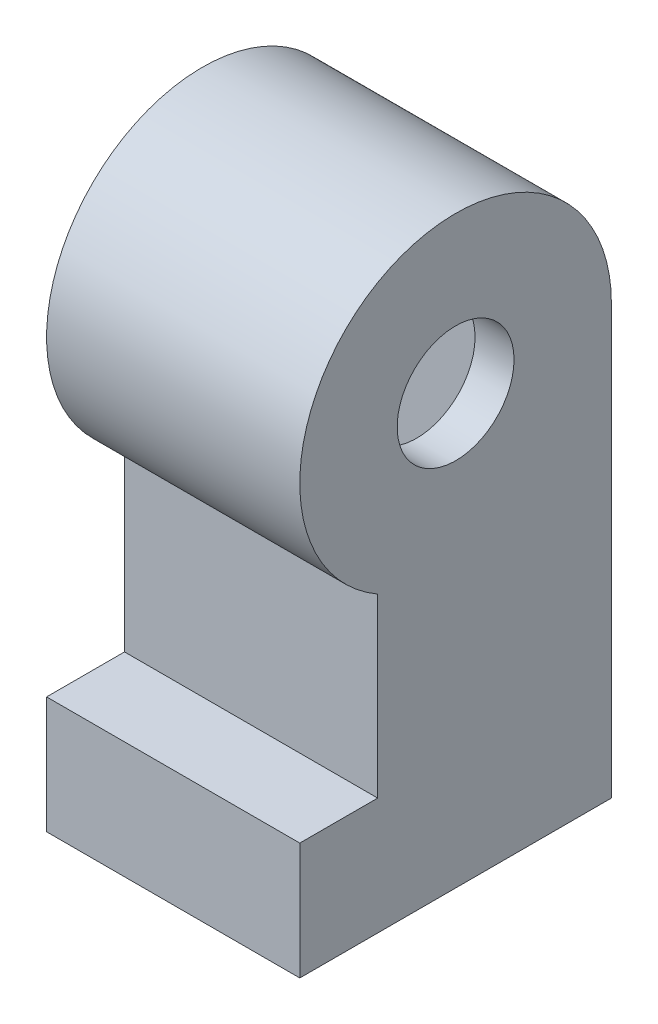
ISO-10303-21;
HEADER;
FILE_DESCRIPTION(('STEP AP214'),'2;1');
FILE_NAME('part.step','',(''),(''),'','','');
FILE_SCHEMA(('AUTOMOTIVE_DESIGN { 1 0 10303 214 1 1 1 1 }'));
ENDSEC;
DATA;
#1=APPLICATION_CONTEXT('core data for automotive mechanical design processes');
#2=APPLICATION_PROTOCOL_DEFINITION('international standard','automotive_design',2000,#1);
#3=PRODUCT_CONTEXT('',#1,'mechanical');
#4=PRODUCT('Part','Part','',(#3));
#5=PRODUCT_RELATED_PRODUCT_CATEGORY('part','',(#4));
#6=PRODUCT_DEFINITION_FORMATION('','',#4);
#7=PRODUCT_DEFINITION_CONTEXT('part definition',#1,'design');
#8=PRODUCT_DEFINITION('design','',#6,#7);
#9=PRODUCT_DEFINITION_SHAPE('','',#8);
#10=(LENGTH_UNIT() NAMED_UNIT(*) SI_UNIT(.MILLI.,.METRE.));
#11=(NAMED_UNIT(*) PLANE_ANGLE_UNIT() SI_UNIT($,.RADIAN.));
#12=(NAMED_UNIT(*) SI_UNIT($,.STERADIAN.) SOLID_ANGLE_UNIT());
#13=UNCERTAINTY_MEASURE_WITH_UNIT(LENGTH_MEASURE(1.E-05),#10,'distance_accuracy_value','');
#14=(GEOMETRIC_REPRESENTATION_CONTEXT(3) GLOBAL_UNCERTAINTY_ASSIGNED_CONTEXT((#13)) GLOBAL_UNIT_ASSIGNED_CONTEXT((#10,
#11,#12)) REPRESENTATION_CONTEXT('',''));
#15=CARTESIAN_POINT('',(0.,0.,0.));
#16=DIRECTION('',(0.,0.,1.));
#17=DIRECTION('',(1.,0.,0.));
#18=AXIS2_PLACEMENT_3D('',#15,#16,#17);
#19=CARTESIAN_POINT('',(6.5,-11.,-4.));
#20=DIRECTION('',(0.,1.,0.));
#21=DIRECTION('',(0.,0.,1.));
#22=AXIS2_PLACEMENT_3D('',#19,#20,#21);
#23=PLANE('',#22);
#24=DIRECTION('',(0.,0.,-1.));
#25=VECTOR('',#24,1.);
#26=CARTESIAN_POINT('',(0.,-11.,-4.));
#27=LINE('',#26,#25);
#28=CARTESIAN_POINT('',(0.,-11.,4.));
#29=VERTEX_POINT('',#28);
#30=CARTESIAN_POINT('',(0.,-11.,-4.));
#31=VERTEX_POINT('',#30);
#32=EDGE_CURVE('E144',#29,#31,#27,.T.);
#33=ORIENTED_EDGE('',*,*,#32,.T.);
#34=DIRECTION('',(-1.,0.,0.));
#35=VECTOR('',#34,1.);
#36=CARTESIAN_POINT('',(6.5,-11.,-4.));
#37=LINE('',#36,#35);
#38=CARTESIAN_POINT('',(6.5,-11.,-4.));
#39=VERTEX_POINT('',#38);
#40=EDGE_CURVE('E126',#39,#31,#37,.T.);
#41=ORIENTED_EDGE('',*,*,#40,.F.);
#42=DIRECTION('',(0.,0.,-1.));
#43=VECTOR('',#42,1.);
#44=CARTESIAN_POINT('',(6.5,-11.,-4.));
#45=LINE('',#44,#43);
#46=CARTESIAN_POINT('',(6.5,-11.,4.));
#47=VERTEX_POINT('',#46);
#48=EDGE_CURVE('E115',#47,#39,#45,.T.);
#49=ORIENTED_EDGE('',*,*,#48,.F.);
#50=DIRECTION('',(-1.,0.,0.));
#51=VECTOR('',#50,1.);
#52=CARTESIAN_POINT('',(6.5,-11.,4.));
#53=LINE('',#52,#51);
#54=EDGE_CURVE('E122',#47,#29,#53,.T.);
#55=ORIENTED_EDGE('',*,*,#54,.T.);
#56=EDGE_LOOP('',(#33,#41,#49,#55));
#57=FACE_BOUND('',#56,.T.);
#58=DIRECTION('',(0.,0.,-1.));
#59=VECTOR('',#58,1.);
#60=CARTESIAN_POINT('',(1.,-11.,-4.));
#61=LINE('',#60,#59);
#62=CARTESIAN_POINT('',(1.,-11.,3.));
#63=VERTEX_POINT('',#62);
#64=CARTESIAN_POINT('',(1.,-11.,-3.));
#65=VERTEX_POINT('',#64);
#66=EDGE_CURVE('E171',#63,#65,#61,.T.);
#67=ORIENTED_EDGE('',*,*,#66,.F.);
#68=DIRECTION('',(-1.,0.,0.));
#69=VECTOR('',#68,1.);
#70=CARTESIAN_POINT('',(6.5,-11.,3.));
#71=LINE('',#70,#69);
#72=CARTESIAN_POINT('',(5.5,-11.,3.));
#73=VERTEX_POINT('',#72);
#74=EDGE_CURVE('E173',#73,#63,#71,.T.);
#75=ORIENTED_EDGE('',*,*,#74,.F.);
#76=DIRECTION('',(0.,0.,-1.));
#77=VECTOR('',#76,1.);
#78=CARTESIAN_POINT('',(5.5,-11.,-4.));
#79=LINE('',#78,#77);
#80=CARTESIAN_POINT('',(5.5,-11.,-3.));
#81=VERTEX_POINT('',#80);
#82=EDGE_CURVE('E53',#73,#81,#79,.T.);
#83=ORIENTED_EDGE('',*,*,#82,.T.);
#84=DIRECTION('',(-1.,0.,0.));
#85=VECTOR('',#84,1.);
#86=CARTESIAN_POINT('',(6.5,-11.,-3.));
#87=LINE('',#86,#85);
#88=EDGE_CURVE('E169',#81,#65,#87,.T.);
#89=ORIENTED_EDGE('',*,*,#88,.T.);
#90=EDGE_LOOP('',(#67,#75,#83,#89));
#91=FACE_BOUND('',#90,.T.);
#92=ADVANCED_FACE('F39',(#57,#91),#23,.F.);
#93=CARTESIAN_POINT('',(6.5,0.,0.));
#94=DIRECTION('',(-1.,0.,0.));
#95=DIRECTION('',(0.,0.,1.));
#96=AXIS2_PLACEMENT_3D('',#93,#94,#95);
#97=CYLINDRICAL_SURFACE('',#96,4.);
#98=CARTESIAN_POINT('',(0.,0.,0.));
#99=DIRECTION('',(1.,0.,0.));
#100=DIRECTION('',(0.,0.,-1.));
#101=AXIS2_PLACEMENT_3D('',#98,#99,#100);
#102=CIRCLE('',#101,4.);
#103=CARTESIAN_POINT('',(0.,0.,-4.));
#104=VERTEX_POINT('',#103);
#105=CARTESIAN_POINT('',(0.,-3.46410161513776,2.));
#106=VERTEX_POINT('',#105);
#107=EDGE_CURVE('E137',#104,#106,#102,.T.);
#108=ORIENTED_EDGE('',*,*,#107,.T.);
#109=DIRECTION('',(-1.,0.,0.));
#110=VECTOR('',#109,1.);
#111=CARTESIAN_POINT('',(6.5,-3.46410161513776,2.));
#112=LINE('',#111,#110);
#113=CARTESIAN_POINT('',(6.5,-3.46410161513776,2.));
#114=VERTEX_POINT('',#113);
#115=EDGE_CURVE('E11',#114,#106,#112,.T.);
#116=ORIENTED_EDGE('',*,*,#115,.F.);
#117=CARTESIAN_POINT('',(6.5,0.,0.));
#118=DIRECTION('',(1.,0.,0.));
#119=DIRECTION('',(0.,0.,-1.));
#120=AXIS2_PLACEMENT_3D('',#117,#118,#119);
#121=CIRCLE('',#120,4.);
#122=CARTESIAN_POINT('',(6.5,0.,-4.));
#123=VERTEX_POINT('',#122);
#124=EDGE_CURVE('E146',#123,#114,#121,.T.);
#125=ORIENTED_EDGE('',*,*,#124,.F.);
#126=DIRECTION('',(-1.,0.,0.));
#127=VECTOR('',#126,1.);
#128=CARTESIAN_POINT('',(6.5,0.,-4.));
#129=LINE('',#128,#127);
#130=EDGE_CURVE('E135',#123,#104,#129,.T.);
#131=ORIENTED_EDGE('',*,*,#130,.T.);
#132=EDGE_LOOP('',(#108,#116,#125,#131));
#133=FACE_BOUND('',#132,.T.);
#134=ADVANCED_FACE('F41',(#133),#97,.T.);
#135=CARTESIAN_POINT('',(6.5,-8.,2.));
#136=DIRECTION('',(0.,0.,-1.));
#137=DIRECTION('',(-1.,0.,0.));
#138=AXIS2_PLACEMENT_3D('',#135,#136,#137);
#139=PLANE('',#138);
#140=DIRECTION('',(0.,-1.,0.));
#141=VECTOR('',#140,1.);
#142=CARTESIAN_POINT('',(0.,-8.,2.));
#143=LINE('',#142,#141);
#144=CARTESIAN_POINT('',(0.,-8.,2.));
#145=VERTEX_POINT('',#144);
#146=EDGE_CURVE('E136',#106,#145,#143,.T.);
#147=ORIENTED_EDGE('',*,*,#146,.T.);
#148=DIRECTION('',(-1.,0.,0.));
#149=VECTOR('',#148,1.);
#150=CARTESIAN_POINT('',(6.5,-8.,2.));
#151=LINE('',#150,#149);
#152=CARTESIAN_POINT('',(6.5,-8.,2.));
#153=VERTEX_POINT('',#152);
#154=EDGE_CURVE('E50',#153,#145,#151,.T.);
#155=ORIENTED_EDGE('',*,*,#154,.F.);
#156=DIRECTION('',(0.,-1.,0.));
#157=VECTOR('',#156,1.);
#158=CARTESIAN_POINT('',(6.5,-8.,2.));
#159=LINE('',#158,#157);
#160=EDGE_CURVE('E98',#114,#153,#159,.T.);
#161=ORIENTED_EDGE('',*,*,#160,.F.);
#162=ORIENTED_EDGE('',*,*,#115,.T.);
#163=EDGE_LOOP('',(#147,#155,#161,#162));
#164=FACE_BOUND('',#163,.T.);
#165=ADVANCED_FACE('F241',(#164),#139,.F.);
#166=CARTESIAN_POINT('',(6.5,-8.,4.));
#167=DIRECTION('',(0.,-1.,0.));
#168=DIRECTION('',(0.,0.,-1.));
#169=AXIS2_PLACEMENT_3D('',#166,#167,#168);
#170=PLANE('',#169);
#171=DIRECTION('',(0.,0.,1.));
#172=VECTOR('',#171,1.);
#173=CARTESIAN_POINT('',(0.,-8.,4.));
#174=LINE('',#173,#172);
#175=CARTESIAN_POINT('',(0.,-8.,4.));
#176=VERTEX_POINT('',#175);
#177=EDGE_CURVE('E142',#145,#176,#174,.T.);
#178=ORIENTED_EDGE('',*,*,#177,.T.);
#179=DIRECTION('',(-1.,0.,0.));
#180=VECTOR('',#179,1.);
#181=CARTESIAN_POINT('',(6.5,-8.,4.));
#182=LINE('',#181,#180);
#183=CARTESIAN_POINT('',(6.5,-8.,4.));
#184=VERTEX_POINT('',#183);
#185=EDGE_CURVE('E130',#184,#176,#182,.T.);
#186=ORIENTED_EDGE('',*,*,#185,.F.);
#187=DIRECTION('',(0.,0.,1.));
#188=VECTOR('',#187,1.);
#189=CARTESIAN_POINT('',(6.5,-8.,4.));
#190=LINE('',#189,#188);
#191=EDGE_CURVE('E113',#153,#184,#190,.T.);
#192=ORIENTED_EDGE('',*,*,#191,.F.);
#193=ORIENTED_EDGE('',*,*,#154,.T.);
#194=EDGE_LOOP('',(#178,#186,#192,#193));
#195=FACE_BOUND('',#194,.T.);
#196=ADVANCED_FACE('F152',(#195),#170,.F.);
#197=CARTESIAN_POINT('',(6.5,-11.,4.));
#198=DIRECTION('',(0.,0.,-1.));
#199=DIRECTION('',(-1.,0.,0.));
#200=AXIS2_PLACEMENT_3D('',#197,#198,#199);
#201=PLANE('',#200);
#202=DIRECTION('',(0.,-1.,0.));
#203=VECTOR('',#202,1.);
#204=CARTESIAN_POINT('',(0.,-11.,4.));
#205=LINE('',#204,#203);
#206=EDGE_CURVE('E121',#176,#29,#205,.T.);
#207=ORIENTED_EDGE('',*,*,#206,.T.);
#208=ORIENTED_EDGE('',*,*,#54,.F.);
#209=DIRECTION('',(0.,-1.,0.));
#210=VECTOR('',#209,1.);
#211=CARTESIAN_POINT('',(6.5,-11.,4.));
#212=LINE('',#211,#210);
#213=EDGE_CURVE('E107',#184,#47,#212,.T.);
#214=ORIENTED_EDGE('',*,*,#213,.F.);
#215=ORIENTED_EDGE('',*,*,#185,.T.);
#216=EDGE_LOOP('',(#207,#208,#214,#215));
#217=FACE_BOUND('',#216,.T.);
#218=ADVANCED_FACE('F124',(#217),#201,.F.);
#219=CARTESIAN_POINT('',(6.5,0.,-4.));
#220=DIRECTION('',(0.,0.,1.));
#221=DIRECTION('',(0.,-1.,0.));
#222=AXIS2_PLACEMENT_3D('',#219,#220,#221);
#223=PLANE('',#222);
#224=DIRECTION('',(0.,1.,0.));
#225=VECTOR('',#224,1.);
#226=CARTESIAN_POINT('',(0.,0.,-4.));
#227=LINE('',#226,#225);
#228=EDGE_CURVE('E89',#31,#104,#227,.T.);
#229=ORIENTED_EDGE('',*,*,#228,.T.);
#230=ORIENTED_EDGE('',*,*,#130,.F.);
#231=DIRECTION('',(0.,1.,0.));
#232=VECTOR('',#231,1.);
#233=CARTESIAN_POINT('',(6.5,0.,-4.));
#234=LINE('',#233,#232);
#235=EDGE_CURVE('E61',#39,#123,#234,.T.);
#236=ORIENTED_EDGE('',*,*,#235,.F.);
#237=ORIENTED_EDGE('',*,*,#40,.T.);
#238=EDGE_LOOP('',(#229,#230,#236,#237));
#239=FACE_BOUND('',#238,.T.);
#240=ADVANCED_FACE('F158',(#239),#223,.F.);
#241=CARTESIAN_POINT('',(6.5,0.,0.));
#242=DIRECTION('',(1.,0.,0.));
#243=DIRECTION('',(0.,0.,-1.));
#244=AXIS2_PLACEMENT_3D('',#241,#242,#243);
#245=PLANE('',#244);
#246=CARTESIAN_POINT('',(6.5,0.,0.));
#247=DIRECTION('',(1.,0.,0.));
#248=DIRECTION('',(0.,0.,-1.));
#249=AXIS2_PLACEMENT_3D('',#246,#247,#248);
#250=CIRCLE('',#249,1.5);
#251=CARTESIAN_POINT('',(6.5,0.,-1.5));
#252=VERTEX_POINT('',#251);
#253=EDGE_CURVE('E217',#252,#252,#250,.T.);
#254=ORIENTED_EDGE('',*,*,#253,.F.);
#255=EDGE_LOOP('',(#254));
#256=FACE_BOUND('',#255,.T.);
#257=ORIENTED_EDGE('',*,*,#124,.T.);
#258=ORIENTED_EDGE('',*,*,#160,.T.);
#259=ORIENTED_EDGE('',*,*,#191,.T.);
#260=ORIENTED_EDGE('',*,*,#213,.T.);
#261=ORIENTED_EDGE('',*,*,#48,.T.);
#262=ORIENTED_EDGE('',*,*,#235,.T.);
#263=EDGE_LOOP('',(#257,#258,#259,#260,#261,#262));
#264=FACE_BOUND('',#263,.T.);
#265=ADVANCED_FACE('F109',(#256,#264),#245,.T.);
#266=CARTESIAN_POINT('',(0.,0.,0.));
#267=DIRECTION('',(1.,0.,0.));
#268=DIRECTION('',(0.,0.,-1.));
#269=AXIS2_PLACEMENT_3D('',#266,#267,#268);
#270=PLANE('',#269);
#271=ORIENTED_EDGE('',*,*,#107,.F.);
#272=ORIENTED_EDGE('',*,*,#228,.F.);
#273=ORIENTED_EDGE('',*,*,#32,.F.);
#274=ORIENTED_EDGE('',*,*,#206,.F.);
#275=ORIENTED_EDGE('',*,*,#177,.F.);
#276=ORIENTED_EDGE('',*,*,#146,.F.);
#277=EDGE_LOOP('',(#271,#272,#273,#274,#275,#276));
#278=FACE_BOUND('',#277,.T.);
#279=ADVANCED_FACE('F160',(#278),#270,.F.);
#280=CARTESIAN_POINT('',(6.5,0.,0.));
#281=DIRECTION('',(-1.,0.,0.));
#282=DIRECTION('',(0.,0.,1.));
#283=AXIS2_PLACEMENT_3D('',#280,#281,#282);
#284=CYLINDRICAL_SURFACE('',#283,3.);
#285=CARTESIAN_POINT('',(1.,0.,0.));
#286=DIRECTION('',(1.,0.,0.));
#287=DIRECTION('',(0.,0.,-1.));
#288=AXIS2_PLACEMENT_3D('',#285,#286,#287);
#289=CIRCLE('',#288,3.);
#290=CARTESIAN_POINT('',(1.,0.,-3.));
#291=VERTEX_POINT('',#290);
#292=CARTESIAN_POINT('',(1.,-2.82842712474619,0.999999999999999));
#293=VERTEX_POINT('',#292);
#294=EDGE_CURVE('E206',#291,#293,#289,.T.);
#295=ORIENTED_EDGE('',*,*,#294,.F.);
#296=DIRECTION('',(-1.,0.,0.));
#297=VECTOR('',#296,1.);
#298=CARTESIAN_POINT('',(6.5,0.,-3.));
#299=LINE('',#298,#297);
#300=CARTESIAN_POINT('',(5.5,0.,-3.));
#301=VERTEX_POINT('',#300);
#302=EDGE_CURVE('E175',#301,#291,#299,.T.);
#303=ORIENTED_EDGE('',*,*,#302,.F.);
#304=CARTESIAN_POINT('',(5.5,0.,0.));
#305=DIRECTION('',(1.,0.,0.));
#306=DIRECTION('',(0.,0.,-1.));
#307=AXIS2_PLACEMENT_3D('',#304,#305,#306);
#308=CIRCLE('',#307,3.);
#309=CARTESIAN_POINT('',(5.5,-2.82842712474619,0.999999999999999));
#310=VERTEX_POINT('',#309);
#311=EDGE_CURVE('E181',#301,#310,#308,.T.);
#312=ORIENTED_EDGE('',*,*,#311,.T.);
#313=DIRECTION('',(-1.,0.,0.));
#314=VECTOR('',#313,1.);
#315=CARTESIAN_POINT('',(5.5,-2.82842712474619,0.999999999999999));
#316=LINE('',#315,#314);
#317=EDGE_CURVE('E138',#310,#293,#316,.T.);
#318=ORIENTED_EDGE('',*,*,#317,.T.);
#319=EDGE_LOOP('',(#295,#303,#312,#318));
#320=FACE_BOUND('',#319,.T.);
#321=ADVANCED_FACE('F234',(#320),#284,.F.);
#322=CARTESIAN_POINT('',(6.5,-8.,0.999999999999999));
#323=DIRECTION('',(0.,0.,-1.));
#324=DIRECTION('',(-1.,0.,0.));
#325=AXIS2_PLACEMENT_3D('',#322,#323,#324);
#326=PLANE('',#325);
#327=DIRECTION('',(0.,-1.,0.));
#328=VECTOR('',#327,1.);
#329=CARTESIAN_POINT('',(1.,-8.,0.999999999999999));
#330=LINE('',#329,#328);
#331=CARTESIAN_POINT('',(1.,-9.,0.999999999999999));
#332=VERTEX_POINT('',#331);
#333=EDGE_CURVE('E200',#293,#332,#330,.T.);
#334=ORIENTED_EDGE('',*,*,#333,.F.);
#335=ORIENTED_EDGE('',*,*,#317,.F.);
#336=DIRECTION('',(0.,-1.,0.));
#337=VECTOR('',#336,1.);
#338=CARTESIAN_POINT('',(5.5,-8.,0.999999999999999));
#339=LINE('',#338,#337);
#340=CARTESIAN_POINT('',(5.5,-9.,0.999999999999999));
#341=VERTEX_POINT('',#340);
#342=EDGE_CURVE('E195',#310,#341,#339,.T.);
#343=ORIENTED_EDGE('',*,*,#342,.T.);
#344=DIRECTION('',(-1.,0.,0.));
#345=VECTOR('',#344,1.);
#346=CARTESIAN_POINT('',(6.5,-9.,0.999999999999999));
#347=LINE('',#346,#345);
#348=EDGE_CURVE('E198',#341,#332,#347,.T.);
#349=ORIENTED_EDGE('',*,*,#348,.T.);
#350=EDGE_LOOP('',(#334,#335,#343,#349));
#351=FACE_BOUND('',#350,.T.);
#352=ADVANCED_FACE('F286',(#351),#326,.T.);
#353=CARTESIAN_POINT('',(6.5,-9.,4.));
#354=DIRECTION('',(0.,-1.,0.));
#355=DIRECTION('',(0.,0.,-1.));
#356=AXIS2_PLACEMENT_3D('',#353,#354,#355);
#357=PLANE('',#356);
#358=DIRECTION('',(0.,0.,1.));
#359=VECTOR('',#358,1.);
#360=CARTESIAN_POINT('',(1.,-9.,4.));
#361=LINE('',#360,#359);
#362=CARTESIAN_POINT('',(1.,-9.,3.));
#363=VERTEX_POINT('',#362);
#364=EDGE_CURVE('E187',#332,#363,#361,.T.);
#365=ORIENTED_EDGE('',*,*,#364,.F.);
#366=ORIENTED_EDGE('',*,*,#348,.F.);
#367=DIRECTION('',(0.,0.,1.));
#368=VECTOR('',#367,1.);
#369=CARTESIAN_POINT('',(5.5,-9.,4.));
#370=LINE('',#369,#368);
#371=CARTESIAN_POINT('',(5.5,-9.,3.));
#372=VERTEX_POINT('',#371);
#373=EDGE_CURVE('E190',#341,#372,#370,.T.);
#374=ORIENTED_EDGE('',*,*,#373,.T.);
#375=DIRECTION('',(-1.,0.,0.));
#376=VECTOR('',#375,1.);
#377=CARTESIAN_POINT('',(6.5,-9.,3.));
#378=LINE('',#377,#376);
#379=EDGE_CURVE('E178',#372,#363,#378,.T.);
#380=ORIENTED_EDGE('',*,*,#379,.T.);
#381=EDGE_LOOP('',(#365,#366,#374,#380));
#382=FACE_BOUND('',#381,.T.);
#383=ADVANCED_FACE('F299',(#382),#357,.T.);
#384=CARTESIAN_POINT('',(6.5,-11.,3.));
#385=DIRECTION('',(0.,0.,-1.));
#386=DIRECTION('',(-1.,0.,0.));
#387=AXIS2_PLACEMENT_3D('',#384,#385,#386);
#388=PLANE('',#387);
#389=DIRECTION('',(0.,-1.,0.));
#390=VECTOR('',#389,1.);
#391=CARTESIAN_POINT('',(1.,-11.,3.));
#392=LINE('',#391,#390);
#393=EDGE_CURVE('E179',#363,#63,#392,.T.);
#394=ORIENTED_EDGE('',*,*,#393,.F.);
#395=ORIENTED_EDGE('',*,*,#379,.F.);
#396=DIRECTION('',(0.,-1.,0.));
#397=VECTOR('',#396,1.);
#398=CARTESIAN_POINT('',(5.5,-11.,3.));
#399=LINE('',#398,#397);
#400=EDGE_CURVE('E170',#372,#73,#399,.T.);
#401=ORIENTED_EDGE('',*,*,#400,.T.);
#402=ORIENTED_EDGE('',*,*,#74,.T.);
#403=EDGE_LOOP('',(#394,#395,#401,#402));
#404=FACE_BOUND('',#403,.T.);
#405=ADVANCED_FACE('F310',(#404),#388,.T.);
#406=CARTESIAN_POINT('',(6.5,0.,-3.));
#407=DIRECTION('',(0.,0.,1.));
#408=DIRECTION('',(0.,-1.,0.));
#409=AXIS2_PLACEMENT_3D('',#406,#407,#408);
#410=PLANE('',#409);
#411=DIRECTION('',(0.,1.,0.));
#412=VECTOR('',#411,1.);
#413=CARTESIAN_POINT('',(1.,0.,-3.));
#414=LINE('',#413,#412);
#415=EDGE_CURVE('E177',#65,#291,#414,.T.);
#416=ORIENTED_EDGE('',*,*,#415,.F.);
#417=ORIENTED_EDGE('',*,*,#88,.F.);
#418=DIRECTION('',(0.,1.,0.));
#419=VECTOR('',#418,1.);
#420=CARTESIAN_POINT('',(5.5,0.,-3.));
#421=LINE('',#420,#419);
#422=EDGE_CURVE('E167',#81,#301,#421,.T.);
#423=ORIENTED_EDGE('',*,*,#422,.T.);
#424=ORIENTED_EDGE('',*,*,#302,.T.);
#425=EDGE_LOOP('',(#416,#417,#423,#424));
#426=FACE_BOUND('',#425,.T.);
#427=ADVANCED_FACE('F317',(#426),#410,.T.);
#428=CARTESIAN_POINT('',(5.5,0.,0.));
#429=DIRECTION('',(1.,0.,0.));
#430=DIRECTION('',(0.,0.,-1.));
#431=AXIS2_PLACEMENT_3D('',#428,#429,#430);
#432=PLANE('',#431);
#433=CARTESIAN_POINT('',(5.5,0.,0.));
#434=DIRECTION('',(1.,0.,0.));
#435=DIRECTION('',(0.,0.,-1.));
#436=AXIS2_PLACEMENT_3D('',#433,#434,#435);
#437=CIRCLE('',#436,1.5);
#438=CARTESIAN_POINT('',(5.5,0.,-1.5));
#439=VERTEX_POINT('',#438);
#440=EDGE_CURVE('E214',#439,#439,#437,.F.);
#441=ORIENTED_EDGE('',*,*,#440,.F.);
#442=EDGE_LOOP('',(#441));
#443=FACE_BOUND('',#442,.T.);
#444=ORIENTED_EDGE('',*,*,#311,.F.);
#445=ORIENTED_EDGE('',*,*,#422,.F.);
#446=ORIENTED_EDGE('',*,*,#82,.F.);
#447=ORIENTED_EDGE('',*,*,#400,.F.);
#448=ORIENTED_EDGE('',*,*,#373,.F.);
#449=ORIENTED_EDGE('',*,*,#342,.F.);
#450=EDGE_LOOP('',(#444,#445,#446,#447,#448,#449));
#451=FACE_BOUND('',#450,.T.);
#452=ADVANCED_FACE('F328',(#443,#451),#432,.F.);
#453=CARTESIAN_POINT('',(1.,0.,0.));
#454=DIRECTION('',(1.,0.,0.));
#455=DIRECTION('',(0.,0.,-1.));
#456=AXIS2_PLACEMENT_3D('',#453,#454,#455);
#457=PLANE('',#456);
#458=ORIENTED_EDGE('',*,*,#294,.T.);
#459=ORIENTED_EDGE('',*,*,#333,.T.);
#460=ORIENTED_EDGE('',*,*,#364,.T.);
#461=ORIENTED_EDGE('',*,*,#393,.T.);
#462=ORIENTED_EDGE('',*,*,#66,.T.);
#463=ORIENTED_EDGE('',*,*,#415,.T.);
#464=EDGE_LOOP('',(#458,#459,#460,#461,#462,#463));
#465=FACE_BOUND('',#464,.T.);
#466=ADVANCED_FACE('F336',(#465),#457,.T.);
#467=CARTESIAN_POINT('',(-0.00100000000000013,0.,0.));
#468=DIRECTION('',(1.,0.,0.));
#469=DIRECTION('',(0.,0.,-1.));
#470=AXIS2_PLACEMENT_3D('',#467,#468,#469);
#471=CYLINDRICAL_SURFACE('',#470,1.5);
#472=CARTESIAN_POINT('',(6.5,0.,-1.5));
#473=CARTESIAN_POINT('',(6.48958333333333,0.,-1.5));
#474=CARTESIAN_POINT('',(6.47916666666667,0.,-1.5));
#475=CARTESIAN_POINT('',(6.45833333333333,0.,-1.5));
#476=CARTESIAN_POINT('',(6.44791666666667,0.,-1.5));
#477=CARTESIAN_POINT('',(6.42708333333333,0.,-1.5));
#478=CARTESIAN_POINT('',(6.41666666666667,0.,-1.5));
#479=CARTESIAN_POINT('',(6.39583333333333,0.,-1.5));
#480=CARTESIAN_POINT('',(6.38541666666667,0.,-1.5));
#481=CARTESIAN_POINT('',(6.36458333333333,0.,-1.5));
#482=CARTESIAN_POINT('',(6.35416666666667,0.,-1.5));
#483=CARTESIAN_POINT('',(6.33333333333333,0.,-1.5));
#484=CARTESIAN_POINT('',(6.32291666666667,0.,-1.5));
#485=CARTESIAN_POINT('',(6.30208333333333,0.,-1.5));
#486=CARTESIAN_POINT('',(6.29166666666667,0.,-1.5));
#487=CARTESIAN_POINT('',(6.27083333333333,0.,-1.5));
#488=CARTESIAN_POINT('',(6.26041666666667,0.,-1.5));
#489=CARTESIAN_POINT('',(6.23958333333333,0.,-1.5));
#490=CARTESIAN_POINT('',(6.22916666666667,0.,-1.5));
#491=CARTESIAN_POINT('',(6.20833333333333,0.,-1.5));
#492=CARTESIAN_POINT('',(6.19791666666667,0.,-1.5));
#493=CARTESIAN_POINT('',(6.17708333333333,0.,-1.5));
#494=CARTESIAN_POINT('',(6.16666666666667,0.,-1.5));
#495=CARTESIAN_POINT('',(6.14583333333333,0.,-1.5));
#496=CARTESIAN_POINT('',(6.13541666666667,0.,-1.5));
#497=CARTESIAN_POINT('',(6.11458333333333,0.,-1.5));
#498=CARTESIAN_POINT('',(6.10416666666667,0.,-1.5));
#499=CARTESIAN_POINT('',(6.08333333333333,0.,-1.5));
#500=CARTESIAN_POINT('',(6.07291666666667,0.,-1.5));
#501=CARTESIAN_POINT('',(6.05208333333333,0.,-1.5));
#502=CARTESIAN_POINT('',(6.04166666666667,0.,-1.5));
#503=CARTESIAN_POINT('',(6.02083333333333,0.,-1.5));
#504=CARTESIAN_POINT('',(6.01041666666667,0.,-1.5));
#505=CARTESIAN_POINT('',(5.98958333333333,0.,-1.5));
#506=CARTESIAN_POINT('',(5.97916666666667,0.,-1.5));
#507=CARTESIAN_POINT('',(5.95833333333333,0.,-1.5));
#508=CARTESIAN_POINT('',(5.94791666666667,0.,-1.5));
#509=CARTESIAN_POINT('',(5.92708333333333,0.,-1.5));
#510=CARTESIAN_POINT('',(5.91666666666667,0.,-1.5));
#511=CARTESIAN_POINT('',(5.89583333333333,0.,-1.5));
#512=CARTESIAN_POINT('',(5.88541666666667,0.,-1.5));
#513=CARTESIAN_POINT('',(5.86458333333333,0.,-1.5));
#514=CARTESIAN_POINT('',(5.85416666666667,0.,-1.5));
#515=CARTESIAN_POINT('',(5.83333333333333,0.,-1.5));
#516=CARTESIAN_POINT('',(5.82291666666667,0.,-1.5));
#517=CARTESIAN_POINT('',(5.80208333333333,0.,-1.5));
#518=CARTESIAN_POINT('',(5.79166666666667,0.,-1.5));
#519=CARTESIAN_POINT('',(5.77083333333333,0.,-1.5));
#520=CARTESIAN_POINT('',(5.76041666666667,0.,-1.5));
#521=CARTESIAN_POINT('',(5.73958333333333,0.,-1.5));
#522=CARTESIAN_POINT('',(5.72916666666667,0.,-1.5));
#523=CARTESIAN_POINT('',(5.70833333333333,0.,-1.5));
#524=CARTESIAN_POINT('',(5.69791666666667,0.,-1.5));
#525=CARTESIAN_POINT('',(5.67708333333333,0.,-1.5));
#526=CARTESIAN_POINT('',(5.66666666666667,0.,-1.5));
#527=CARTESIAN_POINT('',(5.64583333333333,0.,-1.5));
#528=CARTESIAN_POINT('',(5.63541666666667,0.,-1.5));
#529=CARTESIAN_POINT('',(5.61458333333333,0.,-1.5));
#530=CARTESIAN_POINT('',(5.60416666666667,0.,-1.5));
#531=CARTESIAN_POINT('',(5.58333333333333,0.,-1.5));
#532=CARTESIAN_POINT('',(5.57291666666667,0.,-1.5));
#533=CARTESIAN_POINT('',(5.55208333333333,0.,-1.5));
#534=CARTESIAN_POINT('',(5.54166666666667,0.,-1.5));
#535=CARTESIAN_POINT('',(5.52083333333333,0.,-1.5));
#536=CARTESIAN_POINT('',(5.51041666666667,0.,-1.5));
#537=CARTESIAN_POINT('',(5.5,0.,-1.5));
#538=B_SPLINE_CURVE_WITH_KNOTS('',3,(#472,#473,#474,#475,#476,#477,#478,#479,#480,#481,#482,
#483,#484,#485,#486,#487,#488,#489,#490,#491,#492,#493,#494,#495,#496,#497,#498,#499,#500,#501,
#502,#503,#504,#505,#506,#507,#508,#509,#510,#511,#512,#513,#514,#515,#516,#517,#518,#519,#520,
#521,#522,#523,#524,#525,#526,#527,#528,#529,#530,#531,#532,#533,#534,#535,#536,#537),
.UNSPECIFIED.,.F.,.F.,(4,2,2,2,2,2,2,2,2,2,2,2,2,2,2,2,2,2,2,2,2,2,2,2,2,2,2,2,2,2,2,2,4),(0.,
0.03125,0.0625000000000001,0.0937500000000001,0.125,0.15625,0.1875,0.21875,0.25,
0.281249999999999,0.312499999999999,0.343749999999999,0.374999999999999,0.40625,0.4375,0.46875,
0.5,0.53125,0.5625,0.59375,0.625,0.65625,0.6875,0.718749999999999,0.749999999999999,
0.781249999999999,0.812499999999999,0.843749999999999,0.874999999999999,0.906249999999999,
0.937499999999999,0.968749999999999,0.999999999999999),.UNSPECIFIED.);
#539=EDGE_CURVE('BSEAM225',#252,#439,#538,.T.);
#540=ORIENTED_EDGE('',*,*,#253,.T.);
#541=ORIENTED_EDGE('',*,*,#440,.T.);
#542=ORIENTED_EDGE('',*,*,#539,.T.);
#543=ORIENTED_EDGE('',*,*,#539,.F.);
#544=EDGE_LOOP('',(#540,#542,#541,#543));
#545=FACE_BOUND('',#544,.T.);
#546=ADVANCED_FACE('F225',(#545),#471,.F.);
#547=CLOSED_SHELL('',(#92,#134,#165,#196,#218,#240,#265,#279,#321,#352,#383,#405,#427,#452,#466,#546));
#548=MANIFOLD_SOLID_BREP('B2',#547);
#549=ADVANCED_BREP_SHAPE_REPRESENTATION('',(#18,#548),#14);
#550=SHAPE_DEFINITION_REPRESENTATION(#9,#549);
ENDSEC;
END-ISO-10303-21;
